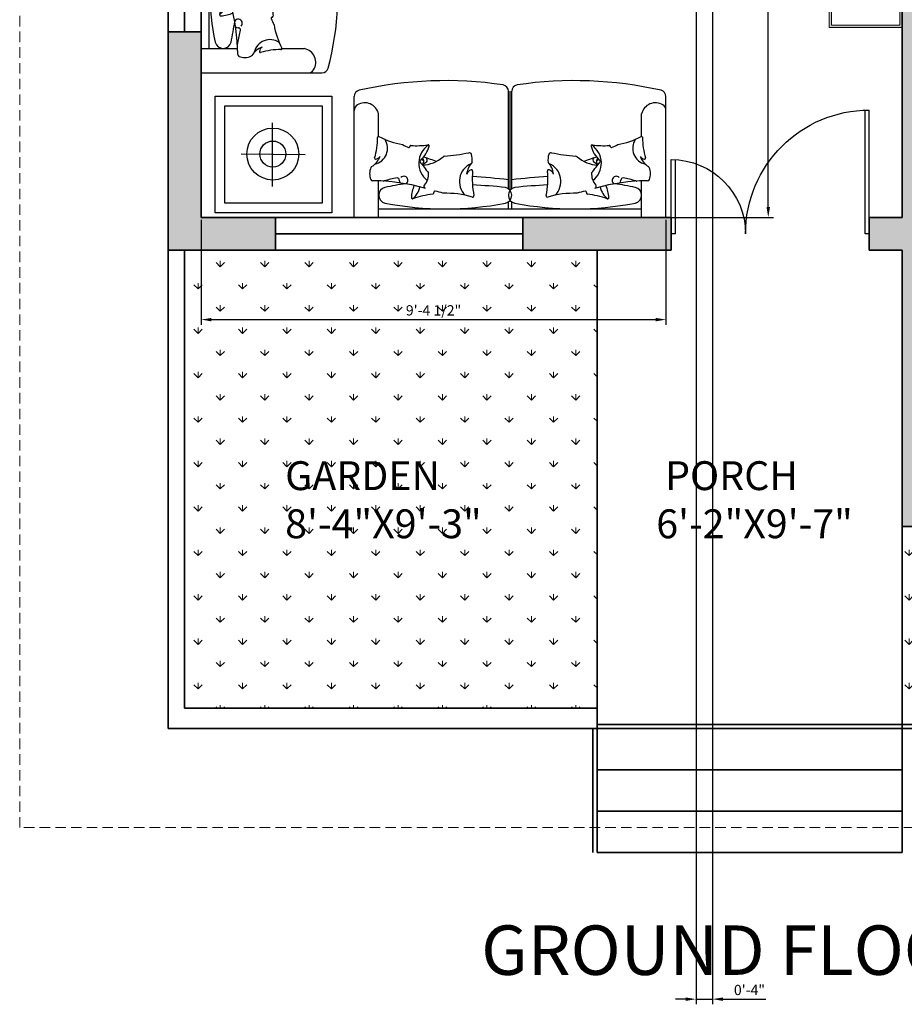
# Model space of a CAD drawing. Units: inches. Extents: x 1566 to 2546, y 1087 to 2705.
# Tile 1 of 27: x 1606 to 1820, y 1087 to 1326. Entities that reach past the tile are written whole.
import ezdxf

# ---------------------------------------------------------------- set-up
doc = ezdxf.new("R2010")
doc.units = ezdxf.units.IN
doc.linetypes.add('DASHED', pattern=[19.05, 12.7, -6.35])
for name, color, linetype, lineweight in [('A-ANNO-DIMS', 2, 'Continuous', 18), ('A-AREA-IDEN', 7, 'Continuous', 18), ('A-DOOR', 4, 'Continuous', 25), ('A-FLOR-OVHD', 8, 'DASHED', 18), ('A-FLOR-PATT', 3, 'Continuous', 13), ('A-FURN', 8, 'Continuous', 18), ('A-WALL', 7, 'Continuous', 35), ('A-WALL-PATT', 8, 'Continuous', 13), ('aparador', 36, 'Continuous', 9), ('moveis', 254, 'Continuous', 5)]:
    doc.layers.add(name, color=color, linetype=linetype, lineweight=lineweight)
for name, color, linetype in [('HID', 11, 'Continuous'), ('SAN', 5, 'Continuous'), ('wood', 26, 'Continuous')]:
    doc.layers.add(name, color=color, linetype=linetype)
doc.styles.get("Standard").update_dxf_attribs({"font": 'arial.ttf'})
doc.dimstyles.new('ISO-25', dxfattribs={"dimtxt": 2.5, "dimasz": 2.5, "dimexe": 1.25, "dimexo": 0.625, "dimtad": 1, "dimtxsty": 'Standard', "dimcen": 2.5, "dimadec": 0, "dimazin": 0, "dimtfac": 1, "dimtmove": 0, "dimatfit": 3, "dimfxl": 1, "dimarcsym": 0})

# ---------------------------------------------------------------- blocks, each defined once
blk = doc.blocks.new('MD')
for p, q in [((1753.46, 1293.03), (1753.46, 1323.03)), ((1754.46, 1293.03), (1754.46, 1323.03)), ((1800.46, 1293.03), (1800.46, 1311.03)), ((1801.46, 1293.03), (1801.46, 1311.03)), ((1753.46, 1293.03), (1754.46, 1293.03)), ((1800.46, 1293.03), (1801.46, 1293.03))]:
    blk.add_line(p, q)
at = {"ltscale": 0.3}
for centre, radius, start, end in [((1753.46, 1293.03), 30, 0, 90), ((1801.46, 1293.03), 18, 90, 180)]:
    blk.add_arc(centre, radius, start, end, dxfattribs=at)
blk = doc.blocks.new('Aparador ORGANICA Formatto')
at = {"layer": 'aparador', "ltscale": 0.3}
h = blk.add_hatch(color=256, dxfattribs=at)
h.dxf.hatch_style = 1
h.set_gradient(color1=(118, 213, 123), color2=(52, 168, 57), one_color=1, tint=0.43, name='INVCURVED')
h.paths.add_polyline_path([(0.8, 0.45), (-0.8, 0.45), (-0.8, 0), (0.8, 0)])
h.paths.add_polyline_path([(0.785, 0.435), (0.785, 0.015), (-0.785, 0.015), (-0.785, 0.435)], flags=16)
h.paths.add_polyline_path([(0.2911, 0.3699), (0.5365, 0.3699), (0.5365, 0.3757), (0.6011, 0.3757), (0.6011, 0.3699), (0.6011, 0.3499), (0.6011, 0.3441), (0.5365, 0.3441), (0.5365, 0.3499), (0.3338, 0.3499, -0.150336), (0.6449, 0.0488), (0.5923, 0.0199, 0.208852), (0.1632, 0.3499), (-0.1632, 0.3499, 0.208852), (-0.5923, 0.0199), (-0.6449, 0.0488, -0.150336), (-0.3338, 0.3499), (-0.5365, 0.3499), (-0.5365, 0.3441), (-0.6011, 0.3441), (-0.6011, 0.3499), (-0.6011, 0.3699), (-0.6011, 0.3757), (-0.5365, 0.3757), (-0.5365, 0.3699), (-0.2911, 0.3699, -0.206106)], flags=0)
h = blk.add_hatch(color=256, dxfattribs=at)
h.dxf.hatch_style = 1
h.set_gradient(color1=(135, 92, 69), color2=(0, 0, 0), one_color=1, name='INVCURVED')
h.paths.add_polyline_path([(-0.6449, 0.0488), (-0.5923, 0.0199, -0.590888), (0.5923, 0.0199), (0.6449, 0.0488, 0.590888)])
h = blk.add_hatch(color=256, dxfattribs=at)
h.dxf.hatch_style = 1
h.set_gradient(color1=(178, 189, 189), one_color=1, tint=1, name='CYLINDER')
h.paths.add_polyline_path([(-0.5365, 0.3757), (-0.6011, 0.3757), (-0.6011, 0.3699), (-0.5365, 0.3699)])
h.paths.add_polyline_path([(-0.5365, 0.3499), (-0.6011, 0.3499), (-0.6011, 0.3441), (-0.5365, 0.3441)])
h = blk.add_hatch(color=256, dxfattribs=at)
h.dxf.hatch_style = 1
h.set_gradient(color1=(118, 213, 123), color2=(31, 101, 35), one_color=1, tint=0.26, name='INVCURVED')
h.paths.add_polyline_path([(-0.2911, 0.3699), (-0.6011, 0.3699), (-0.6011, 0.3499), (-0.3338, 0.3499, -0.015999)])
h = blk.add_hatch(color=256, dxfattribs=at)
h.dxf.hatch_style = 1
h.set_gradient(color1=(118, 213, 123), color2=(31, 101, 35), one_color=1, tint=0.26, name='INVCURVED')
h.paths.add_polyline_path([(-0.1632, 0.3499), (0.1632, 0.3499, 0.122516)])
h = blk.add_hatch(color=256, dxfattribs=at)
h.dxf.hatch_style = 1
h.set_gradient(color1=(118, 213, 123), color2=(31, 101, 35), one_color=1, tint=0.26, name='INVCURVED')
h.paths.add_polyline_path([(0.6011, 0.3699), (0.2911, 0.3699, -0.015999), (0.3338, 0.3499), (0.6011, 0.3499)])
h = blk.add_hatch(color=256, dxfattribs=at)
h.dxf.hatch_style = 1
h.set_gradient(color1=(178, 189, 189), one_color=1, tint=1, name='CYLINDER')
h.paths.add_polyline_path([(0.6011, 0.3757), (0.5365, 0.3757), (0.5365, 0.3699), (0.6011, 0.3699)])
h.paths.add_polyline_path([(0.6011, 0.3499), (0.5365, 0.3499), (0.5365, 0.3441), (0.6011, 0.3441)])
for p, q in [((-0.5923, 0.0199), (-0.6449, 0.0488)), ((0.5923, 0.0199), (0.6449, 0.0488))]:
    blk.add_line(p, q, dxfattribs=at)
for points in [[(-0.6011, 0.3699), (-0.6011, 0.3757), (-0.5365, 0.3757), (-0.5365, 0.3699)], [(0.6011, 0.3699), (0.6011, 0.3757), (0.5365, 0.3757), (0.5365, 0.3699)], [(-0.5365, 0.3499), (-0.5365, 0.3441), (-0.6011, 0.3441), (-0.6011, 0.3499)], [(0.5365, 0.3499), (0.5365, 0.3441), (0.6011, 0.3441), (0.6011, 0.3499)]]:
    blk.add_lwpolyline(points, dxfattribs=at)
for radius in [0.7362, 0.6762]:
    blk.add_arc((0, -0.3063), radius, 28.84335, 151.15665, dxfattribs=at)
at = {"layer": 'moveis', "ltscale": 0.3}
for p, q in [((-0.6011, 0.3699), (-0.6011, 0.3499)), ((-0.2911, 0.3699), (-0.6011, 0.3699)), ((0.2911, 0.3699), (0.6011, 0.3699)), ((0.6011, 0.3699), (0.6011, 0.3499)), ((-0.6011, 0.3499), (-0.3338, 0.3499)), ((-0.1632, 0.3499), (0.1632, 0.3499)), ((0.6011, 0.3499), (0.3338, 0.3499))]:
    blk.add_line(p, q, dxfattribs=at)
for points in [[(-0.8, 0), (0.8, 0), (0.8, 0.45), (-0.8, 0.45)], [(-0.785, 0.015), (0.785, 0.015), (0.785, 0.435), (-0.785, 0.435)]]:
    blk.add_lwpolyline(points, close=True, dxfattribs=at)
blk = doc.blocks.new('123')
at = {"layer": 'HID'}
for centre, radius, start, end in [((1246.02, 1434.08), 0.283, 70.5302, 181.6176), ((1253.29, 1434.28), 7.55, 181.6176, 204.8398), ((1243.23, 1430.56), 4.68, 10.8696, 54.3073), ((1254.03, 1456.71), 23.73, 250.5302, 262.522), ((1250.9, 1432.91), 0.283, 348.0525, 82.522), ((1251.46, 1432.79), 0.283, 168.0525, 279.4331), ((1249.65, 1443.68), 11.32, 279.4331, 289.3248), ((1254.03, 1456.71), 23.73, 268.4714, 286.0168), ((1262.09, 1430.12), 4.71, 134.8494, 245.9788), ((1279.38, 1429.58), 18.88, 167.7826, 186.0053), ((1260.65, 1433.64), 0.283, 347.7826, 106.0168), ((1278.71, 1433.64), 0.283, 73.9832, 192.2174), ((1259.98, 1429.58), 18.88, 353.9947, 12.2174), ((1285.34, 1456.71), 23.73, 253.9832, 271.5286), ((1277.28, 1430.12), 4.71, 294.0212, 45.1506), ((1289.72, 1443.68), 11.32, 250.6752, 260.5669), ((1287.91, 1432.79), 0.283, 260.5669, 11.9475), ((1288.46, 1432.91), 0.283, 97.478, 191.9475), ((1285.34, 1456.71), 23.73, 277.478, 289.4698), ((1296.13, 1430.56), 4.68, 125.6927, 169.1304), ((1286.07, 1434.28), 7.55, 335.1602, 358.3824), ((1293.34, 1434.08), 0.283, 358.3824, 109.4698), ((1235.86, 1479.09), 49.13, 270.5535, 285.4148), ((1243.86, 1429.85), 1.05, 142.8444, 177.2985), ((1243.92, 1429.87), 0.999, 224.2238, 57.6435), ((1249.25, 1431.33), 0.472, 105.6578, 222.8337), ((1246.1, 1428.4), 3.83, 354.2387, 42.8337), ((1293.27, 1428.4), 3.83, 137.1663, 185.7613), ((1290.11, 1431.33), 0.472, 317.1663, 74.3422), ((1303.5, 1479.09), 49.13, 254.5852, 269.4465), ((1295.45, 1429.87), 0.999, 122.3565, 315.7762), ((1295.5, 1429.85), 1.05, 2.7015, 37.1556), ((1239.48, 1428.24), 3.85, 158.334, 202.6623), ((1236.34, 1429.49), 0.472, 90.5535, 158.334), ((1235.86, 1479.09), 49.13, 270.5535, 273.614), ((1238.99, 1429.59), 0.472, 66.2045, 93.614), ((1245.71, 1450.89), 21.87, 252.6177, 260.951), ((1242.35, 1429.76), 0.472, 260.951, 7.3574), ((1243.29, 1429.88), 0.472, 177.2985, 187.3574), ((1252.86, 1425.7), 5.32, 127.6048, 236.1053), ((1285.54, 1398.1), 46.53, 139.9755, 144.1671), ((1260.85, 1429.07), 1.87, 202.9525, 250.443), ((1264.95, 1429.26), 5.89, 188.9571, 220.4913), ((1274.42, 1429.26), 5.89, 319.5087, 351.0429), ((1278.51, 1429.07), 1.87, 289.557, 337.0475), ((1253.83, 1398.1), 46.53, 35.8329, 40.0245), ((1286.5, 1425.7), 5.32, 303.8947, 52.3952), ((1297.02, 1429.76), 0.472, 172.6426, 279.049), ((1296.08, 1429.88), 0.472, 352.6426, 2.7015), ((1293.65, 1450.89), 21.87, 279.049, 287.3823), ((1300.38, 1429.59), 0.472, 86.386, 113.7955), ((1303.5, 1479.09), 49.13, 266.386, 269.4465), ((1303.02, 1429.49), 0.472, 21.666, 89.4465), ((1299.88, 1428.24), 3.85, 337.3377, 21.666), ((1236.36, 1426.94), 0.472, 202.6623, 238.3929), ((1233.54, 1422.36), 4.91, 20.2155, 58.3929), ((1236.02, 1422.11), 3.93, 326.1078, 77.2372), ((1247.81, 1425.22), 0.945, 310.8427, 57.338), ((1253.61, 1432.21), 7.94, 229.38, 238.0577), ((1248.02, 1418.03), 8.16, 48.6039, 87.0681), ((1260.32, 1427.58), 0.283, 250.443, 6.0053), ((1279.04, 1427.58), 0.283, 173.9947, 289.557), ((1291.34, 1418.03), 8.16, 92.9319, 131.3961), ((1285.75, 1432.21), 7.94, 301.9423, 310.62), ((1291.56, 1425.22), 0.945, 122.662, 229.1573), ((1303.34, 1422.11), 3.93, 102.7628, 213.8922), ((1305.82, 1422.36), 4.91, 121.6071, 159.7845), ((1303, 1426.94), 0.472, 301.6071, 337.3377), ((1237.05, 1424.48), 0.236, 81.7015, 197.2637), ((1221.8, 1419.74), 15.74, 359.041, 17.2637), ((1236.86, 1423.18), 1.56, 34.2109, 81.7015), ((1248.01, 1425.2), 0.236, 144.1671, 251.1685), ((1243.89, 1420.15), 6.29, 12.876, 50.0789), ((1227.67, 1473.6), 52.85, 292.7112, 293.5018), ((1268.16, 1374.24), 53.54, 107.709, 111.2519), ((1248.79, 1424.95), 0.814, 313.9174, 40.1627), ((1253.8, 1424.57), 0.567, 227.5655, 264.8479), ((1248.46, 1365.29), 58.96, 79.0518, 84.8479), ((1259.76, 1423.73), 0.567, 259.0518, 342.8696), ((1256.05, 1424.88), 4.45, 342.8696, 7.2038), ((1283.31, 1424.88), 4.45, 172.7962, 197.1304), ((1279.6, 1423.73), 0.567, 197.1304, 280.9482), ((1290.9, 1365.29), 58.96, 95.1521, 100.9482), ((1285.56, 1424.57), 0.567, 275.1521, 312.4345), ((1271.2, 1374.24), 53.54, 68.7481, 72.291), ((1295.47, 1420.15), 6.29, 129.9211, 167.124), ((1290.58, 1424.95), 0.814, 139.8373, 226.0826), ((1311.69, 1473.6), 52.85, 246.4982, 247.2888), ((1291.36, 1425.2), 0.236, 288.8315, 35.8329), ((1302.5, 1423.18), 1.56, 98.2985, 145.7891), ((1317.56, 1419.74), 15.74, 162.7363, 180.959), ((1302.31, 1424.48), 0.236, 342.7363, 98.2985), ((1246.94, 1401.69), 19.77, 99.7298, 117.2752), ((1248.4, 1413.06), 9.43, 110.6915, 120.5832), ((1245.15, 1421.66), 0.236, 359.311, 110.6915), ((1245.62, 1421.66), 0.236, 179.311, 273.7804), ((1246.94, 1401.69), 19.77, 81.7886, 93.7804), ((1249.8, 1421.5), 0.236, 261.7886, 12.876), ((1249.8, 1421.5), 0.236, 261.7886, 12.876), ((1289.57, 1421.5), 0.236, 167.124, 278.2114), ((1289.57, 1421.5), 0.236, 167.124, 278.2114), ((1292.43, 1401.69), 19.77, 86.2196, 98.2114), ((1293.75, 1421.66), 0.236, 266.2196, 0.689), ((1294.22, 1421.66), 0.236, 69.3085, 180.689), ((1290.97, 1413.06), 9.43, 59.4168, 69.3085), ((1292.43, 1401.69), 19.77, 62.7248, 80.2702), ((1237.77, 1419.48), 0.236, 179.041, 297.2752), ((1301.6, 1419.48), 0.236, 242.7248, 0.959), ((1183.3, 1391.63), 19.77, 348.4714, 6.0168), ((1203.2, 1393.73), 0.236, 67.7826, 186.0168), ((1206.29, 1394.4), 3.93, 214.8494, 325.9788), ((1209.24, 1408.51), 15.74, 247.7826, 266.0053), ((1206.97, 1393.23), 1.56, 282.9525, 330.443), ((1207.41, 1396.62), 4.91, 268.9571, 300.4913), ((1208.12, 1392.58), 0.236, 330.443, 86.0053), ((1209.72, 1388.68), 3.71, 62.8696, 87.2038), ((1257.53, 1373.83), 49.13, 159.0518, 164.8479), ((1211.2, 1391.57), 0.472, 339.0518, 62.8696), ((1193.36, 1386.15), 9.43, 359.4331, 9.3248), ((1183.3, 1391.63), 19.77, 330.5302, 342.522), ((1202.38, 1385.62), 0.236, 68.0525, 162.522), ((1202.56, 1386.06), 0.236, 248.0525, 359.4331), ((1213.67, 1381.56), 6.13, 127.5655, 169.079), ((1199.58, 1383.44), 9.43, 359.0692, 11.4619), ((1209.64, 1386.8), 0.472, 307.5655, 344.8479), ((1203.21, 1378.98), 3.9, 356.4825, 134.3073), ((1204.32, 1386.81), 5.27, 309.1869, 318.5341), ((1191.35, 1384.83), 17.84, 340.6607, 353.8744), ((1208.63, 1383.01), 0.472, 349.5475, 138.5341), ((1200.72, 1381.79), 0.236, 150.5302, 261.6176), ((1201.6, 1387.78), 6.29, 261.6176, 299.5758), ((1204.83, 1382.1), 0.236, 32.8897, 119.5758), ((1165.95, 1356.96), 46.53, 28.8632, 32.8897), ((1207.62, 1379.5), 0.917, 184.9476, 286.1991), ((1207.74, 1379.07), 0.472, 286.1991, 340.6607), ((1187.51, 1377.19), 19.77, 328.4714, 346.0168), ((1210.06, 1371.93), 3.93, 194.8494, 305.9788), ((1206.93, 1372.36), 0.236, 47.7826, 166.0168), ((1217.66, 1384.18), 15.74, 227.7826, 246.0053), ((1210.31, 1370.6), 1.56, 262.9525, 310.443), ((1211.88, 1373.63), 4.91, 248.9571, 280.4913), ((1211.17, 1369.59), 0.236, 310.443, 66.0053), ((1211.34, 1365.39), 3.71, 42.8696, 67.2038), ((1195.1, 1368.6), 9.43, 339.4331, 349.3248), ((1251.18, 1335.08), 49.13, 139.0518, 144.8479), ((1213.71, 1367.59), 0.472, 319.0518, 42.8696), ((1187.51, 1377.19), 19.77, 310.5302, 322.522), ((1203.39, 1365.02), 0.236, 48.0525, 142.522), ((1203.71, 1365.37), 0.236, 228.0525, 339.4331), ((1200.52, 1361.98), 0.236, 130.5302, 241.6176), ((1201.9, 1358.5), 3.9, 336.4825, 114.3073), ((1203.4, 1367.31), 6.29, 241.6176, 279.5758), ((1204.48, 1360.87), 0.236, 12.8897, 99.5758), ((1212.61, 1357.35), 6.13, 107.5655, 149.079), ((1200.01, 1363.93), 9.43, 339.0692, 351.4619), ((1210.62, 1363.64), 0.472, 287.5655, 324.8479), ((1181.91, 1357.9), 19.77, 349.7298, 7.2752), ((1201.76, 1360.43), 0.236, 69.041, 187.2752), ((1204.83, 1361.17), 3.93, 216.1078, 327.2372), ((1207.47, 1375.34), 15.74, 249.041, 267.2637), ((1159.36, 1350.55), 46.53, 8.8632, 12.8897), ((1205.91, 1363.41), 4.91, 270.2155, 308.3929), ((1205.54, 1360.02), 1.56, 284.2109, 331.7015), ((1192.75, 1368.04), 17.84, 320.6607, 333.8744), ((1206.71, 1359.39), 0.236, 331.7015, 87.2637), ((1205.62, 1365.47), 5.27, 289.1869, 298.5341), ((1208.36, 1360.43), 0.472, 329.5475, 118.5341), ((1209.25, 1359.2), 0.472, 92.6623, 128.3929), ((1209.41, 1355.82), 3.85, 48.334, 92.6623), ((1211.66, 1358.35), 0.472, 340.5535, 48.334), ((1206.22, 1357.48), 0.917, 164.9476, 266.1991), ((1206.19, 1357.03), 0.472, 266.1991, 320.6607), ((1258.43, 1341.83), 49.13, 160.5535, 175.4148), ((1258.43, 1341.83), 49.13, 160.5535, 163.614), ((1192.09, 1352.64), 9.43, 0.6915, 10.5832), ((1228.56, 1342.22), 21.87, 142.6177, 150.951), ((1210.84, 1355.82), 0.472, 316.2045, 343.614), ((1181.91, 1357.9), 19.77, 331.7886, 343.7804), ((1201.12, 1352.31), 0.236, 69.311, 163.7804), ((1201.29, 1352.75), 0.236, 249.311, 0.6915), ((1209.42, 1351.1), 0.999, 114.2238, 307.6435), ((1209.85, 1352.61), 0.472, 150.951, 257.3574), ((1209.65, 1351.69), 0.472, 67.2985, 77.3574), ((1209.42, 1351.16), 1.05, 32.8444, 67.2985), ((1202.44, 1344.12), 5.32, 17.6048, 126.1053), ((1199.54, 1348.44), 0.236, 151.7886, 262.876), ((1199.54, 1348.44), 0.236, 151.7886, 262.876), ((1200.29, 1354.45), 6.29, 262.876, 300.0789), ((1203.73, 1349.03), 0.945, 200.8427, 307.338), ((1256.07, 1351.41), 52.85, 182.7112, 183.5018), ((1203.63, 1348.85), 0.236, 34.1671, 141.1685), ((1165.33, 1322.86), 46.53, 29.9755, 34.1671), ((1155.85, 1369.08), 52.85, 337.2794, 337.2982), ((1207.3, 1349.55), 3.83, 244.2387, 292.8337), ((1208.97, 1345.59), 0.472, 355.6578, 112.8337), ((1199.97, 1337.3), 0.283, 77.7826, 196.0168), ((1176.89, 1330.67), 23.73, 358.4714, 16.0168), ((1204.03, 1356.03), 18.88, 257.7826, 276.0053), ((1206.03, 1336.97), 0.283, 340.443, 96.0053), ((1203.48, 1338.74), 4.71, 224.8494, 335.9788), ((1204.35, 1341.6), 5.89, 278.9571, 310.4913), ((1204.54, 1337.5), 1.87, 292.9525, 340.443), ((1208.73, 1332.7), 4.45, 72.8696, 97.2038), ((1268.32, 1325.11), 58.96, 169.0518, 174.8479), ((1209.88, 1336.41), 0.567, 349.0518, 72.8696), ((1189.93, 1326.3), 11.32, 9.4331, 19.3248), ((1215.58, 1324.67), 8.16, 138.6039, 177.0681), ((1209.03, 1330.45), 0.567, 317.5655, 354.8479), ((1200.7, 1327.55), 0.283, 78.0525, 172.522), ((1200.82, 1328.1), 0.283, 258.0525, 9.4331), ((1259.37, 1344.81), 53.54, 197.709, 201.2519), ((1176.89, 1330.67), 23.73, 340.5302, 352.522), ((1202.28, 1325.9), 0.472, 195.6578, 312.8337), ((1154.52, 1312.51), 49.13, 0.5535, 15.4148), ((1205.2, 1322.75), 3.83, 84.2387, 132.8337), ((1207.91, 1329.51), 5.32, 217.6048, 326.1053), ((1235.51, 1362.19), 46.53, 229.9755, 234.1671), ((1201.4, 1330.26), 7.94, 319.38, 328.0577), ((1208.38, 1324.46), 0.945, 40.8427, 147.338), ((1208.66, 1325.44), 0.814, 43.9174, 130.1627), ((1160.01, 1304.32), 52.85, 22.7112, 23.5018), ((1213.46, 1320.54), 6.29, 102.876, 140.0789), ((1212.11, 1326.45), 0.236, 351.7886, 102.876), ((1212.11, 1326.45), 0.236, 351.7886, 102.876), ((1231.92, 1323.59), 19.77, 171.7886, 183.7804), ((1203.05, 1319.88), 4.68, 100.8696, 144.3073), ((1199.33, 1329.94), 7.55, 271.6176, 294.8398), ((1208.41, 1324.65), 0.236, 234.1671, 341.1685), ((1199.53, 1322.67), 0.283, 160.5302, 271.6176), ((1203.74, 1320.57), 0.999, 314.2238, 147.6435), ((1211.95, 1321.8), 0.236, 89.311, 200.6915), ((1220.55, 1325.05), 9.43, 200.6915, 210.5832), ((1211.95, 1322.27), 0.236, 269.311, 3.7804), ((1203.76, 1320.51), 1.05, 232.8444, 267.2985), ((1182.72, 1322.36), 21.87, 342.6177, 350.951), ((1203.73, 1319.94), 0.472, 267.2985, 277.3574), ((1203.85, 1319), 0.472, 350.951, 97.3574), ((1231.92, 1323.59), 19.77, 189.7298, 207.2752), ((1204.02, 1315.64), 0.472, 156.2045, 183.614), ((1211.49, 1312.67), 3.93, 56.1078, 167.2372), ((1154.52, 1312.51), 49.13, 0.5535, 3.614), ((1211.25, 1310.19), 4.91, 110.2155, 148.3929), ((1210.43, 1313.51), 1.56, 124.2109, 171.7015), ((1209.12, 1313.7), 0.236, 171.7015, 287.2637), ((1213.86, 1298.45), 15.74, 89.041, 107.2637), ((1214.13, 1314.42), 0.236, 269.041, 27.2752), ((1204.12, 1312.99), 0.472, 180.5535, 248.334), ((1205.37, 1316.13), 3.85, 248.334, 292.6623), ((1206.67, 1313.01), 0.472, 292.6623, 328.3929), ((1221.8, 1292.6), 15.74, 342.7363, 0.959), ((1236.02, 1290.24), 3.93, 282.7628, 33.8922), ((1237.77, 1292.87), 0.236, 62.7248, 180.959), ((1246.94, 1310.66), 19.77, 242.7248, 260.2702), ((1292.43, 1310.66), 19.77, 279.7298, 297.2752), ((1303.34, 1290.24), 3.93, 146.1078, 257.2372), ((1301.6, 1292.87), 0.236, 359.041, 117.2752), ((1317.56, 1292.6), 15.74, 179.041, 197.2637), ((1248.4, 1299.29), 9.43, 239.4168, 249.3085), ((1245.15, 1290.69), 0.236, 249.3085, 0.689), ((1245.62, 1290.69), 0.236, 86.2196, 180.689), ((1246.94, 1310.66), 19.77, 266.2196, 278.2114), ((1252.86, 1286.65), 5.32, 123.8947, 232.3952), ((1243.89, 1292.2), 6.29, 309.9211, 347.124), ((1249.8, 1290.85), 0.236, 347.124, 98.2114), ((1249.8, 1290.85), 0.236, 347.124, 98.2114), ((1289.57, 1290.85), 0.236, 81.7886, 192.876), ((1289.57, 1290.85), 0.236, 81.7886, 192.876), ((1295.47, 1292.2), 6.29, 192.876, 230.0789), ((1286.5, 1286.65), 5.32, 307.6048, 56.1053), ((1292.43, 1310.66), 19.77, 261.7886, 273.7804), ((1293.75, 1290.69), 0.236, 359.311, 93.7804), ((1294.22, 1290.69), 0.236, 179.311, 290.6915), ((1290.97, 1299.29), 9.43, 290.6915, 300.5832), ((1233.54, 1289.99), 4.91, 301.6071, 339.7845), ((1237.05, 1287.87), 0.236, 162.7363, 278.2985), ((1236.86, 1289.17), 1.56, 278.2985, 325.7891), ((1248.01, 1287.15), 0.236, 108.8315, 215.8329), ((1227.67, 1238.75), 52.85, 66.4982, 67.2888), ((1247.81, 1287.12), 0.945, 302.662, 49.1573), ((1248.02, 1294.32), 8.16, 272.9319, 311.3961), ((1268.16, 1338.11), 53.54, 248.7481, 252.291), ((1248.79, 1287.4), 0.814, 319.8373, 46.0826), ((1253.8, 1287.77), 0.567, 95.1521, 132.4345), ((1248.46, 1347.06), 58.96, 275.1521, 280.9482), ((1259.76, 1288.62), 0.567, 17.1304, 100.9482), ((1256.05, 1287.47), 4.45, 352.7962, 17.1304), ((1283.31, 1287.47), 4.45, 162.8696, 187.2038), ((1279.6, 1288.62), 0.567, 79.0518, 162.8696), ((1290.9, 1347.06), 58.96, 259.0518, 264.8479), ((1285.56, 1287.77), 0.567, 47.5655, 84.8479), ((1291.34, 1294.32), 8.16, 228.6039, 267.0681), ((1271.2, 1338.11), 53.54, 287.709, 291.2519), ((1290.58, 1287.4), 0.814, 133.9174, 220.1627), ((1291.56, 1287.12), 0.945, 130.8427, 237.338), ((1311.69, 1238.75), 52.85, 112.7112, 113.5018), ((1291.36, 1287.15), 0.236, 324.1671, 71.1685), ((1302.5, 1289.17), 1.56, 214.2109, 261.7015), ((1305.82, 1289.99), 4.91, 200.2155, 238.3929), ((1302.31, 1287.87), 0.236, 261.7015, 17.2637), ((1239.48, 1284.11), 3.85, 157.3377, 201.666), ((1236.36, 1285.41), 0.472, 121.6071, 157.3377), ((1285.54, 1314.25), 46.53, 215.8329, 220.0245), ((1253.61, 1280.14), 7.94, 121.9423, 130.62), ((1262.09, 1282.22), 4.71, 114.0212, 225.1506), ((1264.95, 1283.09), 5.89, 139.5087, 171.0429), ((1260.85, 1283.28), 1.87, 109.557, 157.0475), ((1260.32, 1284.77), 0.283, 353.9947, 109.557), ((1279.38, 1282.77), 18.88, 173.9947, 192.2174), ((1259.98, 1282.77), 18.88, 347.7826, 6.0053), ((1279.04, 1284.77), 0.283, 70.443, 186.0053), ((1274.42, 1283.09), 5.89, 8.9571, 40.4913), ((1278.51, 1283.28), 1.87, 22.9525, 70.443), ((1277.28, 1282.22), 4.71, 314.8494, 65.9788), ((1253.83, 1314.25), 46.53, 319.9755, 324.1671), ((1285.75, 1280.14), 7.94, 49.38, 58.0577), ((1303, 1285.41), 0.472, 22.6623, 58.3929), ((1299.88, 1284.11), 3.85, 338.334, 22.6623), ((1236.34, 1282.86), 0.472, 201.666, 269.4465), ((1235.86, 1233.26), 49.13, 74.5852, 89.4465), ((1235.86, 1233.26), 49.13, 86.386, 89.4465), ((1238.99, 1282.76), 0.472, 266.386, 293.7955), ((1245.71, 1261.46), 21.87, 99.049, 107.3823), ((1242.35, 1282.59), 0.472, 352.6426, 99.049), ((1243.29, 1282.47), 0.472, 172.6426, 182.7015), ((1243.86, 1282.5), 1.05, 182.7015, 217.1556), ((1243.92, 1282.48), 0.999, 302.3565, 135.7762), ((1246.1, 1283.94), 3.83, 317.1663, 5.7613), ((1293.27, 1283.94), 3.83, 174.2387, 222.8337), ((1303.5, 1233.26), 49.13, 90.5535, 105.4148), ((1295.45, 1282.48), 0.999, 44.2238, 237.6435), ((1295.5, 1282.5), 1.05, 322.8444, 357.2985), ((1297.02, 1282.59), 0.472, 80.951, 187.3574), ((1296.08, 1282.47), 0.472, 357.2985, 7.3574), ((1293.65, 1261.46), 21.87, 72.6177, 80.951), ((1300.38, 1282.76), 0.472, 246.2045, 273.614), ((1303.5, 1233.26), 49.13, 90.5535, 93.614), ((1303.02, 1282.86), 0.472, 270.5535, 338.334), ((1253.29, 1278.07), 7.55, 155.1602, 178.3824), ((1243.23, 1281.79), 4.68, 305.6927, 349.1304), ((1249.25, 1281.02), 0.472, 137.1663, 254.3422), ((1290.11, 1281.02), 0.472, 285.6578, 42.8337), ((1296.13, 1281.79), 4.68, 190.8696, 234.3073), ((1286.07, 1278.07), 7.55, 1.6176, 24.8398), ((1246.02, 1278.27), 0.283, 178.3824, 289.4698), ((1254.03, 1255.63), 23.73, 97.478, 109.4698), ((1250.9, 1279.44), 0.283, 277.478, 11.9475), ((1251.46, 1279.56), 0.283, 80.5669, 191.9475), ((1249.65, 1268.67), 11.32, 70.6752, 80.5669), ((1254.03, 1255.63), 23.73, 73.9832, 91.5286), ((1260.65, 1278.71), 0.283, 253.9832, 12.2174), ((1278.71, 1278.71), 0.283, 167.7826, 286.0168), ((1285.34, 1255.63), 23.73, 88.4714, 106.0168), ((1289.72, 1268.67), 11.32, 99.4331, 109.3248), ((1287.91, 1279.56), 0.283, 348.0525, 99.4331), ((1288.46, 1279.44), 0.283, 168.0525, 262.522), ((1285.34, 1255.63), 23.73, 70.5302, 82.522), ((1293.34, 1278.27), 0.283, 250.5302, 1.6176)]:
    blk.add_arc(centre, radius, start, end, dxfattribs=at)
at = {"layer": 'SAN'}
for p, q in [((1212.06, 1431.34), (1212.06, 1415.9)), ((1220, 1423.66), (1204.47, 1423.49)), ((1212.06, 1281.01), (1212.06, 1296.45)), ((1220, 1288.69), (1204.47, 1288.86))]:
    blk.add_line(p, q, dxfattribs=at)
for centre, radius in [((1212.15, 1423.49), 6.3), ((1212.15, 1423.49), 3.15), ((1212.15, 1288.86), 6.3), ((1212.15, 1288.86), 3.15)]:
    blk.add_circle(centre, radius, dxfattribs=at)
at = {"layer": 'wood'}
for p, q in [((1307.48, 1438.84), (1231.89, 1438.84)), ((1231.89, 1438.84), (1231.89, 1409.55)), ((1237.79, 1438.84), (1237.79, 1430)), ((1301.57, 1438.84), (1301.57, 1430)), ((1307.48, 1438.84), (1307.48, 1409.55)), ((1301.57, 1436.87), (1237.79, 1436.87)), ((1269.29, 1436.87), (1269.29, 1435.11)), ((1270.08, 1436.87), (1270.08, 1435.11)), ((1269.29, 1431.89), (1269.29, 1408.27)), ((1269.68, 1431.89), (1269.68, 1408.27)), ((1270.08, 1431.89), (1270.08, 1408.27)), ((1237.79, 1419.24), (1237.79, 1413.76)), ((1301.57, 1419.24), (1301.57, 1413.76)), ((1194.77, 1308.54), (1194.77, 1403.81)), ((1194.77, 1403.81), (1224.06, 1403.81)), ((1194.77, 1397.91), (1219.85, 1397.91)), ((1196.74, 1314.44), (1196.74, 1397.91)), ((1196.74, 1371.13), (1198.49, 1371.13)), ((1201.72, 1371.13), (1225.34, 1371.13)), ((1196.74, 1370.35), (1225.34, 1370.35)), ((1196.74, 1369.56), (1225.34, 1369.56)), ((1196.74, 1342.79), (1198.49, 1342.79)), ((1196.74, 1342), (1225.34, 1342)), ((1201.72, 1342.79), (1225.34, 1342.79)), ((1196.74, 1341.21), (1198.49, 1341.21)), ((1201.72, 1341.21), (1225.34, 1341.21)), ((1194.77, 1314.44), (1203.61, 1314.44)), ((1214.37, 1314.44), (1219.85, 1314.44)), ((1194.77, 1308.54), (1224.06, 1308.54)), ((1269.29, 1280.46), (1269.29, 1304.08)), ((1269.68, 1280.46), (1269.68, 1304.08)), ((1270.08, 1280.46), (1270.08, 1304.08)), ((1231.89, 1273.51), (1231.89, 1302.8)), ((1307.48, 1273.51), (1307.48, 1302.8)), ((1237.79, 1293.11), (1237.79, 1298.59)), ((1301.57, 1293.11), (1301.57, 1298.59)), ((1237.79, 1273.51), (1237.79, 1282.35)), ((1301.57, 1273.51), (1301.57, 1282.35)), ((1301.57, 1275.48), (1237.79, 1275.48)), ((1269.29, 1275.48), (1269.29, 1277.24)), ((1270.08, 1275.48), (1270.08, 1277.24)), ((1307.48, 1273.51), (1231.89, 1273.51))]:
    blk.add_line(p, q, dxfattribs=at)
for points in [[(1198.13, 1409.44), (1226.48, 1409.44), (1226.48, 1437.78), (1198.13, 1437.78)], [(1200.49, 1411.8), (1224.11, 1411.8), (1224.11, 1435.42), (1200.49, 1435.42)], [(1198.13, 1302.91), (1226.48, 1302.91), (1226.48, 1274.57), (1198.13, 1274.57)], [(1200.49, 1300.55), (1224.11, 1300.55), (1224.11, 1276.93), (1200.49, 1276.93)]]:
    blk.add_lwpolyline(points, close=True, dxfattribs=at)
for centre, radius, start, end in [((1239.8, 1433.5), 1.97, 104.0803, 255.9197), ((1253.99, 1357.1), 79.67, 79.4658, 100.6108), ((1268.09, 1433.5), 1.98, 283.4421, 76.5579), ((1271.27, 1433.5), 1.98, 103.4421, 256.5579), ((1285.38, 1357.1), 79.67, 79.3892, 100.5342), ((1299.57, 1433.5), 1.97, 284.0803, 75.9197), ((1251.62, 1486.43), 56.2, 257.3591, 262.5789), ((1239.14, 1754.92), 324.68, 273.7815, 275.1985), ((1300.23, 1754.92), 324.68, 264.8015, 266.2185), ((1287.75, 1486.43), 56.2, 277.4211, 282.6409), ((1241.58, 1693.38), 265.11, 274.0948, 275.9995), ((1297.79, 1693.38), 265.11, 264.0005, 265.9052), ((1234.43, 1414.5), 3.44, 238.6411, 347.5888), ((1304.93, 1414.5), 3.44, 192.4112, 301.3589), ((1233.46, 1412.91), 1.57, 180, 238.6411), ((1305.9, 1412.91), 1.57, 301.3589, 0), ((1233.46, 1409.55), 1.57, 180, 255.2393), ((1305.9, 1409.55), 1.57, 284.7607, 0), ((1254.02, 1500.46), 94.78, 257.2232, 278.4687), ((1267.71, 1408.27), 1.57, 279.7794, 0), ((1271.65, 1408.27), 1.57, 180, 260.2206), ((1285.34, 1500.46), 94.78, 261.5313, 282.7768), ((1219.11, 1401.27), 3.44, 282.4112, 31.3589), ((1220.7, 1402.24), 1.57, 31.3589, 90), ((1224.06, 1402.24), 1.57, 14.7607, 90), ((1156.82, 1384.52), 71.11, 350.2206, 14.7607), ((1200.11, 1395.9), 1.97, 14.0803, 165.9197), ((1147.18, 1384.08), 58.17, 9.2978, 13.7486), ((1253.04, 1384.08), 56.2, 167.3591, 192.5496), ((1147.18, 1384.08), 56.2, 6.399, 12.6409), ((1147.18, 1384.08), 56.2, 347.4504, 357.5986), ((1147.18, 1384.08), 58.17, 347.1404, 357.743), ((1200.11, 1372.33), 1.98, 193.4421, 346.5579), ((1225.34, 1372.71), 1.57, 270, 350.2206), ((1200.11, 1367.56), 1.97, 14.0803, 165.9197), ((1147.18, 1355.74), 58.17, 10.7847, 13.7486), ((1225.34, 1367.99), 1.57, 9.7794, 90), ((1156.82, 1356.17), 71.11, 350.2206, 9.7794), ((1253.04, 1355.74), 56.2, 167.3591, 192.5496), ((1147.18, 1355.74), 56.2, 8.9885, 12.6409), ((1147.18, 1355.74), 56.2, 4.5548, 5.3997), ((1147.18, 1355.74), 56.2, 347.4504, 352.6454), ((1147.18, 1355.74), 58.17, 347.1404, 351.9048), ((1200.11, 1343.98), 1.98, 193.4421, 346.5579), ((1200.11, 1340.02), 1.98, 13.4421, 166.5579), ((1225.34, 1344.36), 1.57, 270, 350.2206), ((1253.04, 1328.27), 56.2, 167.4504, 192.6409), ((1147.18, 1328.27), 56.2, 9.1435, 12.5496), ((1147.18, 1328.27), 58.17, 8.7934, 12.8596), ((1225.34, 1339.64), 1.57, 9.7794, 90), ((1156.82, 1327.83), 71.11, 345.2393, 9.7794), ((1147.18, 1328.27), 56.2, 347.3591, 352.5789), ((1200.11, 1316.45), 1.97, 194.0803, 345.9197), ((1219.11, 1311.08), 3.44, 328.6411, 77.5888), ((1220.7, 1310.11), 1.57, 270, 328.6411), ((1224.06, 1310.11), 1.57, 270, 345.2393), ((1254.02, 1211.88), 94.78, 81.5313, 102.7768), ((1285.34, 1211.88), 94.78, 77.2232, 98.4687), ((1233.46, 1302.8), 1.57, 104.7607, 180), ((1267.71, 1304.08), 1.57, 0, 80.2206), ((1271.65, 1304.08), 1.57, 99.7794, 180), ((1305.9, 1302.8), 1.57, 0, 75.2393), ((1233.46, 1299.44), 1.57, 121.3589, 180), ((1234.43, 1297.85), 3.44, 12.4112, 121.3589), ((1304.93, 1297.85), 3.44, 58.6411, 167.5888), ((1305.9, 1299.44), 1.57, 0, 58.6411), ((1241.58, 1018.97), 265.11, 84.0005, 85.9052), ((1297.79, 1018.97), 265.11, 94.0948, 95.9995), ((1239.8, 1278.85), 1.97, 104.0803, 255.9197), ((1251.62, 1225.92), 56.2, 97.4211, 102.6409), ((1239.14, 957.43), 324.68, 84.8015, 86.2185), ((1268.09, 1278.85), 1.98, 283.4421, 76.5579), ((1271.27, 1278.85), 1.98, 103.4421, 256.5579), ((1300.23, 957.43), 324.68, 93.7815, 95.1985), ((1287.75, 1225.92), 56.2, 77.3591, 82.5789), ((1299.57, 1278.85), 1.97, 284.0803, 75.9197), ((1253.99, 1355.25), 79.67, 259.3892, 280.5342), ((1285.38, 1355.25), 79.67, 259.4658, 280.6108)]:
    blk.add_arc(centre, radius, start, end, dxfattribs=at)
blk = doc.blocks.new('*D61')
at = {"layer": 'A-ANNO-DIMS', "color": 0, "lineweight": -2, "transparency": 16777216}
for p, q in [((1762.86, 1443.53), (1788.29, 1443.53)), ((1787.04, 1280.7), (1787.04, 1441.03)), ((1762.86, 1278.2), (1788.29, 1278.2))]:
    blk.add_line(p, q, dxfattribs=at)
at = {"layer": 'A-ANNO-DIMS', "color": 0, "transparency": 16777216}
for points in [[(1786.62, 1441.03), (1787.46, 1441.03), (1787.04, 1443.53)], [(1786.62, 1280.7), (1787.46, 1280.7), (1787.04, 1278.2)]]:
    blk.add_solid(points, dxfattribs=at)
at = {"layer": 'Defpoints', "color": 0, "transparency": 16777216}
for p in [(1762.24, 1443.53), (1787.04, 1443.53), (1762.24, 1278.2)]:
    blk.add_point(p, dxfattribs=at)
at = {"layer": 'A-ANNO-DIMS', "color": 0, "transparency": 16777216, "insert": (1785.12, 1360.86), "char_height": 2.5, "attachment_point": 5, "rotation": 90}
blk.add_mtext('SOFA SET 13\'-9 1/2"', dxfattribs=at)
blk = doc.blocks.new('*D62')
at = {"layer": 'A-ANNO-DIMS', "color": 0, "lineweight": -2, "transparency": 16777216}
for p, q in [((1649.53, 1277.57), (1649.53, 1252.15)), ((1762.24, 1277.57), (1762.24, 1252.15)), ((1652.03, 1253.4), (1759.74, 1253.4))]:
    blk.add_line(p, q, dxfattribs=at)
at = {"layer": 'A-ANNO-DIMS', "color": 0, "transparency": 16777216}
for points in [[(1652.03, 1253.81), (1652.03, 1252.98), (1649.53, 1253.4)], [(1759.74, 1253.81), (1759.74, 1252.98), (1762.24, 1253.4)]]:
    blk.add_solid(points, dxfattribs=at)
at = {"layer": 'Defpoints', "color": 0, "transparency": 16777216}
for p in [(1649.53, 1278.2), (1762.24, 1278.2), (1762.24, 1253.4)]:
    blk.add_point(p, dxfattribs=at)
at = {"layer": 'A-ANNO-DIMS', "color": 0, "transparency": 16777216, "insert": (1705.88, 1255.32), "char_height": 2.5, "attachment_point": 5}
blk.add_mtext('9\'-4 1/2"', dxfattribs=at)
blk = doc.blocks.new('*D110')
at = {"layer": 'A-ANNO-DIMS', "color": 0, "lineweight": -2, "transparency": 16777216}
for p, q in [((1769.53, 1769.57), (1769.53, 1087.35)), ((1773.53, 1769.57), (1773.53, 1087.35)), ((1767.03, 1088.6), (1764.53, 1088.6)), ((1769.53, 1088.6), (1773.53, 1088.6)), ((1776.03, 1088.6), (1786.43, 1088.6))]:
    blk.add_line(p, q, dxfattribs=at)
at = {"layer": 'A-ANNO-DIMS', "color": 0, "transparency": 16777216}
for points in [[(1767.03, 1089.01), (1767.03, 1088.18), (1769.53, 1088.6)], [(1776.03, 1089.01), (1776.03, 1088.18), (1773.53, 1088.6)]]:
    blk.add_solid(points, dxfattribs=at)
at = {"layer": 'Defpoints', "color": 0, "transparency": 16777216}
for p in [(1769.53, 1770.2), (1773.53, 1770.2), (1773.53, 1088.6)]:
    blk.add_point(p, dxfattribs=at)
at = {"layer": 'A-ANNO-DIMS', "color": 0, "transparency": 16777216, "insert": (1782.48, 1090.5), "char_height": 2.5, "attachment_point": 5}
blk.add_mtext('0\'-4"', dxfattribs=at)

msp = doc.modelspace()

# ---------------------------------------------------------------- hatches: boundary and pattern name
at = {"layer": 'A-FLOR-PATT'}
h = msp.add_hatch(dxfattribs=at)
h.set_pattern_fill('GRASS', color=256, scale=0.3)
h.paths.add_polyline_path([(1745.53, 1270.2), (1645.53, 1270.2), (1645.53, 1159.2), (1745.53, 1159.2)])
h.paths.add_polyline_path([(1993.53, 1203.2), (1819.53, 1203.2), (1819.53, 1155.2), (1993.53, 1155.2)])
h.paths.add_polyline_path([(1667.62, 1196.42), (1716.72, 1196.42), (1716.72, 1222.54), (1667.62, 1222.54)], flags=24)
h.paths.add_polyline_path([(1881.06, 1171.45), (1935.47, 1171.45), (1935.47, 1197.57), (1881.06, 1197.57)], flags=24)
at = {"layer": 'A-WALL-PATT'}
h = msp.add_hatch(color=256, dxfattribs=at)
h.dxf.hatch_style = 1
h.paths.add_polyline_path([(2001.53, 1778.2), (1641.53, 1778.2), (1641.53, 1746.2), (1649.53, 1746.2), (1649.53, 1770.2), (1769.53, 1770.2), (1769.53, 1650.2), (1767.53, 1650.2), (1767.53, 1648.2), (1767.53, 1646.2), (1819.53, 1646.2), (1819.53, 1650.2), (1773.53, 1650.2), (1773.53, 1770.2), (1941.53, 1770.2), (1941.53, 1756.2), (1945.53, 1756.2), (1945.53, 1770.2), (1993.53, 1770.2), (1993.53, 1650.2), (1945.53, 1650.2), (1945.53, 1652.2), (1943.53, 1652.2), (1941.53, 1652.2), (1941.53, 1650.2), (1867.53, 1650.2), (1867.53, 1642.2), (1871.53, 1642.2), (1871.53, 1646.2), (1993.53, 1646.2), (1993.53, 1526.2), (1871.53, 1526.2), (1871.53, 1606.2), (1867.53, 1606.2), (1867.53, 1522.2), (1993.53, 1522.2), (1993.53, 1387.2), (1959.53, 1387.2), (1959.53, 1397.2), (1955.53, 1397.2), (1955.53, 1387.2), (1903.53, 1387.2), (1903.53, 1383.2), (1993.53, 1383.2), (1993.53, 1364.3), (1993.53, 1211.2), (1939.53, 1211.2), (1939.53, 1203.2), (1993.53, 1203.2), (1993.53, 1154.2), (2001.53, 1154.2)])
h.paths.add_polyline_path([(1649.53, 1646.2), (1731.53, 1646.2), (1731.53, 1650.2), (1649.53, 1650.2), (1649.53, 1674.2), (1641.53, 1674.2), (1641.53, 1622.2), (1649.53, 1622.2)], flags=17)
h.paths.add_polyline_path([(1649.53, 1550.2), (1641.53, 1550.2), (1641.53, 1510.2), (1649.53, 1510.2), (1649.53, 1522.2), (1731.53, 1522.2), (1731.53, 1500.2), (1735.53, 1500.2), (1735.53, 1522.2), (1767.53, 1522.2), (1767.53, 1500.2), (1771.53, 1500.2), (1771.53, 1526.2), (1649.53, 1526.2)], flags=17)
h.paths.add_polyline_path([(1649.53, 1464.2), (1735.53, 1464.2), (1735.53, 1470.2), (1731.53, 1470.2), (1731.53, 1468.2), (1649.53, 1468.2), (1649.53, 1480.2), (1641.53, 1480.2), (1641.53, 1419.2), (1649.53, 1419.2)], flags=17)
h.paths.add_polyline_path([(1649.53, 1323.2), (1641.53, 1323.2), (1641.53, 1270.2), (1667.53, 1270.2), (1667.53, 1278.2), (1649.53, 1278.2)], flags=17)
h.paths.add_polyline_path([(1763.53, 1278.2), (1727.53, 1278.2), (1727.53, 1270.2), (1763.53, 1270.2)], flags=17)
h.paths.add_polyline_path([(1823.53, 1383.2), (1827.53, 1383.2), (1827.53, 1385.2), (1827.53, 1387.2), (1819.53, 1387.2), (1819.53, 1324.21), (1819.53, 1278.2), (1811.53, 1278.2), (1811.53, 1274.2), (1811.53, 1270.2), (1819.53, 1270.2), (1819.53, 1203.2), (1877.53, 1203.2), (1877.53, 1211.2), (1823.53, 1211.2)], flags=17)

# ---------------------------------------------------------------- linework, layer by layer
at = {"layer": 'A-FLOR-OVHD', "ltscale": 0.2}
for p, q in [((1605.53, 1130.2), (1605.53, 1778.2)), ((2001.53, 1130.2), (1605.53, 1130.2))]:
    msp.add_line(p, q, dxfattribs=at)
at = {"layer": 'A-WALL'}
for p, q in [((1641.53, 1154.2), (1641.53, 1778.2)), ((1649.53, 1278.2), (1649.53, 1464.2)), ((1645.53, 1419.2), (1645.53, 1323.2)), ((1819.53, 1278.2), (1819.53, 1387.2)), ((1649.53, 1323.2), (1641.53, 1323.2)), ((1649.53, 1278.2), (1763.53, 1278.2)), ((1667.53, 1270.2), (1667.53, 1278.2)), ((1727.53, 1270.2), (1727.53, 1278.2)), ((1763.53, 1270.2), (1763.53, 1278.2)), ((1811.53, 1270.2), (1811.53, 1278.2)), ((1811.53, 1278.2), (1819.53, 1278.2)), ((1727.53, 1274.2), (1667.53, 1274.2)), ((1641.53, 1270.2), (1763.53, 1270.2)), ((1645.53, 1159.2), (1645.53, 1270.2)), ((1745.53, 1154.2), (1745.53, 1270.2)), ((1811.53, 1270.2), (1819.53, 1270.2)), ((1819.53, 1155.2), (1819.53, 1270.2)), ((1819.53, 1203.2), (1993.53, 1203.2)), ((1645.53, 1159.2), (1745.53, 1159.2)), ((2001.53, 1154.2), (1641.53, 1154.2)), ((1744.53, 1154.2), (1744.53, 1124.2)), ((1993.53, 1155.2), (1745.53, 1155.2)), ((1745.53, 1154.2), (1745.53, 1124.2)), ((1819.53, 1155.2), (1819.53, 1124.2)), ((1819.53, 1144.2), (1745.53, 1144.2)), ((1819.53, 1134.2), (1745.53, 1134.2)), ((1819.53, 1124.2), (1745.53, 1124.2))]:
    msp.add_line(p, q, dxfattribs=at)

# ---------------------------------------------------------------- block references
at = {"layer": 'A-DOOR', "xscale": -1}
msp.add_blockref('MD', (3564.99, -18.83), dxfattribs=at)
at = {"layer": 'A-FURN'}
msp.add_blockref('123', (454.76, 4.69), dxfattribs=at)
at = {"layer": 'A-FURN', "xscale": 39.3701, "yscale": 39.3701, "zscale": 39.3701, "rotation": 270}
msp.add_blockref('Aparador ORGANICA Formatto', (1801.81, 1355.7), dxfattribs=at)

# ---------------------------------------------------------------- texts
at = {"layer": 'A-AREA-IDEN', "attachment_point": 1}
for s, width, insert, char_height in [('GARDEN\\P8\'-4"X9\'-3"', 111.7553, (1669.9, 1219.05), 7), (' PORCH\\P6\'-2"X9\'-7"', 111.7553, (1759.88, 1219.05), 7), ('GROUND FLOOR PLAN', 267.5424, (1717.44, 1106.48), 12)]:
    msp.add_mtext_dynamic_manual_height_columns(s, width=width, gutter_width=12.5, heights=[0], dxfattribs=dict(at, insert=insert, char_height=char_height))

# ---------------------------------------------------------------- dimensions: what is measured, and where the dimension line sits
at = {"layer": 'A-ANNO-DIMS'}
for base, p1, p2, override, picture, middle in [((1773.53, 1088.6), (1769.53, 1770.2), (1773.53, 1770.2), {"dimdec": 1, "dimlfac": 1, "dimrnd": 0, "dimzin": 1, "dimdsep": 46, "dimlunit": 4, "dimfrac": 2}, '*D110', (1782.48, 1090.5)), ((1762.24, 1253.4), (1649.53, 1278.2), (1762.24, 1278.2), {"dimdec": 1, "dimrnd": 0, "dimzin": 1, "dimlunit": 4, "dimfrac": 2}, '*D62', (1705.88, 1255.32))]:
    dim = msp.add_linear_dim(base=base, p1=p1, p2=p2, dimstyle='ISO-25', override=override, dxfattribs=at)
    dim.commit()
    dim.dimension.update_dxf_attribs({"geometry": picture, "text_midpoint": middle})
dim = msp.add_linear_dim(base=(1787.04, 1443.53), p1=(1762.24, 1278.2), p2=(1762.24, 1443.53), angle=90, text='SOFA SET <>', dimstyle='ISO-25', override={"dimdec": 1, "dimrnd": 0, "dimzin": 1, "dimlunit": 4, "dimfrac": 2}, dxfattribs=at)
dim.commit()
dim.dimension.update_dxf_attribs({"geometry": '*D61', "text_midpoint": (1785.12, 1360.86)})

doc.saveas('drawing.dxf')
